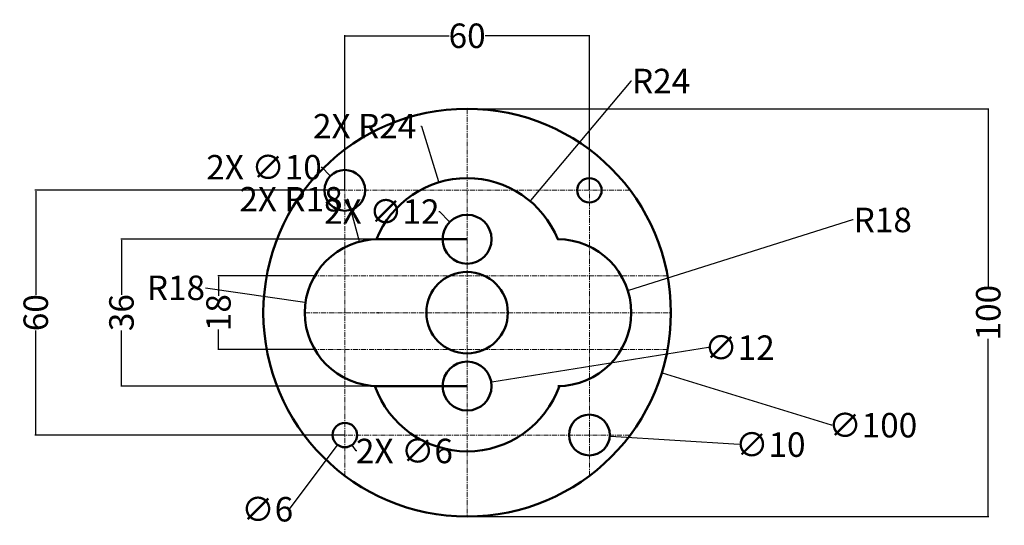
# Model space of a CAD drawing. Units: millimetres. Extents: x -18 to 223, y 11 to 135.
import ezdxf

# ---------------------------------------------------------------- set-up
doc = ezdxf.new("R2010")
doc.units = ezdxf.units.MM
doc.header["$MEASUREMENT"] = 0
doc.linetypes.add('CENTER', pattern=[2, 1.25, -0.25, 0.25, -0.25])
for name, color, linetype, lineweight in [('M-CNTR', 4, 'CENTER', 18), ('M-DIMS', 2, 'Continuous', 25), ('M-OUTL', 7, 'Continuous', 50)]:
    doc.layers.add(name, color=color, linetype=linetype, lineweight=lineweight)
doc.styles.get("Standard").update_dxf_attribs({"font": 'arial.ttf'})
doc.dimstyles.get("Standard").update_dxf_attribs({"dimtxt": 6, "dimasz": 0.18, "dimexe": 0.18, "dimexo": 0.0625, "dimgap": 0.09, "dimtad": 0, "dimtoh": 1, "dimdec": 0, "dimzin": 0, "dimdsep": 46, "dimtxsty": 'Standard', "dimcen": 0.09, "dimadec": 0, "dimazin": 0, "dimtfac": 1, "dimtdec": 0, "dimtofl": 0, "dimtmove": 0, "dimatfit": 3, "dimfxl": 1, "dimtolj": 1, "dimtzin": 0, "dimarcsym": 0})

# ---------------------------------------------------------------- blocks, each defined once
blk = doc.blocks.new('*D1')
at = {"layer": 'Defpoints', "color": 0, "transparency": 16777216}
for p in [(121.61, 131.04), (61.61, 93.14), (121.61, 93.14)]:
    blk.add_point(p, dxfattribs=at)
at = {"layer": 'M-DIMS', "color": 0, "lineweight": -2, "transparency": 16777216}
for p, q in [((61.61, 93.2), (61.61, 131.22)), ((61.79, 131.04), (87.22, 131.04)), ((121.43, 131.04), (96, 131.04)), ((121.61, 93.2), (121.61, 131.22))]:
    blk.add_line(p, q, dxfattribs=at)
at = {"layer": 'M-DIMS', "color": 0, "transparency": 16777216}
for points in [[(61.79, 131.07), (61.79, 131.01), (61.61, 131.04)], [(121.43, 131.07), (121.43, 131.01), (121.61, 131.04)]]:
    blk.add_solid(points, dxfattribs=at)
at = {"layer": 'M-DIMS', "color": 0, "transparency": 16777216, "insert": (91.61, 131.04), "char_height": 6, "attachment_point": 5}
blk.add_mtext('\\A1;60', dxfattribs=at)
blk = doc.blocks.new('*D2')
at = {"layer": 'Defpoints', "color": 0, "transparency": 16777216}
for p in [(43.84, 77.89), (139.39, 48.39)]:
    blk.add_point(p, dxfattribs=at)
at = {"layer": 'M-DIMS', "color": 0, "lineweight": -2, "transparency": 16777216}
for p, q in [((91.52, 63.14), (91.7, 63.14)), ((91.61, 63.05), (91.61, 63.23)), ((180.99, 35.55), (139.56, 48.34)), ((181.17, 35.55), (180.99, 35.55))]:
    blk.add_line(p, q, dxfattribs=at)
at = {"layer": 'M-DIMS', "color": 0, "transparency": 16777216}
blk.add_solid([(139.57, 48.36), (139.55, 48.31), (139.39, 48.39)], dxfattribs=at)
at = {"layer": 'M-DIMS', "color": 0, "transparency": 16777216, "insert": (191.14, 35.55), "char_height": 6, "attachment_point": 5}
blk.add_mtext('\\A1;∅100', dxfattribs=at)
blk = doc.blocks.new('*D3')
at = {"layer": 'Defpoints', "color": 0, "transparency": 16777216}
for p in [(91.61, 113.14), (91.61, 13.14), (219.47, 13.14)]:
    blk.add_point(p, dxfattribs=at)
at = {"layer": 'M-DIMS', "color": 0, "lineweight": -2, "transparency": 16777216}
for p, q in [((91.67, 113.14), (219.65, 113.14)), ((219.47, 112.96), (219.47, 69.56)), ((219.47, 13.32), (219.47, 56.71)), ((91.67, 13.14), (219.65, 13.14))]:
    blk.add_line(p, q, dxfattribs=at)
at = {"layer": 'M-DIMS', "color": 0, "transparency": 16777216}
for points in [[(219.44, 112.96), (219.5, 112.96), (219.47, 113.14)], [(219.44, 13.32), (219.5, 13.32), (219.47, 13.14)]]:
    blk.add_solid(points, dxfattribs=at)
at = {"layer": 'M-DIMS', "color": 0, "transparency": 16777216, "insert": (219.47, 63.14), "char_height": 6, "attachment_point": 5, "rotation": 90}
blk.add_mtext('\\A1;100', dxfattribs=at)
blk = doc.blocks.new('*D4')
at = {"layer": 'Defpoints', "color": 0, "transparency": 16777216}
for p in [(107.05, 90.51), (91.61, 72.14)]:
    blk.add_point(p, dxfattribs=at)
at = {"layer": 'M-DIMS', "color": 0, "lineweight": -2, "transparency": 16777216}
for p, q in [((131.79, 119.94), (107.17, 90.65)), ((131.97, 119.94), (131.79, 119.94)), ((91.52, 72.14), (91.7, 72.14)), ((91.61, 72.05), (91.61, 72.23))]:
    blk.add_line(p, q, dxfattribs=at)
at = {"layer": 'M-DIMS', "color": 0, "transparency": 16777216}
blk.add_solid([(107.14, 90.67), (107.19, 90.63), (107.05, 90.51)], dxfattribs=at)
at = {"layer": 'M-DIMS', "color": 0, "transparency": 16777216, "insert": (139.21, 119.94), "char_height": 6, "attachment_point": 5}
blk.add_mtext('\\A1;R24', dxfattribs=at)
blk = doc.blocks.new('*D5')
at = {"layer": 'Defpoints', "color": 0, "transparency": 16777216}
for p in [(51.98, 65.7), (69.79, 63.14)]:
    blk.add_point(p, dxfattribs=at)
at = {"layer": 'M-DIMS', "color": 0, "lineweight": -2, "transparency": 16777216}
for p, q in [((27.43, 69.23), (51.8, 65.72)), ((69.7, 63.14), (69.88, 63.14)), ((69.79, 63.05), (69.79, 63.23))]:
    blk.add_line(p, q, dxfattribs=at)
at = {"layer": 'M-DIMS', "color": 0, "transparency": 16777216}
blk.add_solid([(51.8, 65.75), (51.79, 65.7), (51.98, 65.7)], dxfattribs=at)
at = {"layer": 'M-DIMS', "color": 0, "transparency": 16777216, "insert": (20.17, 69.23), "char_height": 6, "attachment_point": 5}
blk.add_mtext('\\A1;R18', dxfattribs=at)
blk = doc.blocks.new('*D6')
at = {"layer": 'Defpoints', "color": 0, "transparency": 16777216}
for p in [(131.03, 68.54), (113.86, 63.14)]:
    blk.add_point(p, dxfattribs=at)
at = {"layer": 'M-DIMS', "color": 0, "lineweight": -2, "transparency": 16777216}
for p, q in [((186.14, 85.87), (131.2, 68.59)), ((186.32, 85.87), (186.14, 85.87)), ((113.77, 63.14), (113.95, 63.14)), ((113.86, 63.05), (113.86, 63.23))]:
    blk.add_line(p, q, dxfattribs=at)
at = {"layer": 'M-DIMS', "color": 0, "transparency": 16777216}
blk.add_solid([(131.19, 68.62), (131.21, 68.56), (131.03, 68.54)], dxfattribs=at)
at = {"layer": 'M-DIMS', "color": 0, "transparency": 16777216, "insert": (193.59, 85.87), "char_height": 6, "attachment_point": 5}
blk.add_mtext('\\A1;R18', dxfattribs=at)
blk = doc.blocks.new('*D7')
at = {"layer": 'Defpoints', "color": 0, "transparency": 16777216}
for p in [(63.4, 35.55), (59.82, 30.73)]:
    blk.add_point(p, dxfattribs=at)
at = {"layer": 'M-DIMS', "color": 0, "lineweight": -2, "transparency": 16777216}
for p, q in [((61.52, 33.14), (61.7, 33.14)), ((61.61, 33.05), (61.61, 33.23)), ((48.07, 14.94), (59.71, 30.59)), ((47.89, 14.94), (48.07, 14.94))]:
    blk.add_line(p, q, dxfattribs=at)
at = {"layer": 'M-DIMS', "color": 0, "transparency": 16777216}
blk.add_solid([(59.69, 30.61), (59.74, 30.57), (59.82, 30.73)], dxfattribs=at)
at = {"layer": 'M-DIMS', "color": 0, "transparency": 16777216, "insert": (42.57, 14.94), "char_height": 6, "attachment_point": 5}
blk.add_mtext('\\A1;∅6', dxfattribs=at)
blk = doc.blocks.new('*D8')
at = {"layer": 'Defpoints', "color": 0, "transparency": 16777216}
for p in [(116.62, 33.46), (126.6, 32.82)]:
    blk.add_point(p, dxfattribs=at)
at = {"layer": 'M-DIMS', "color": 0, "lineweight": -2, "transparency": 16777216}
for p, q in [((121.52, 33.14), (121.7, 33.14)), ((121.61, 33.05), (121.61, 33.23)), ((158.37, 30.79), (126.78, 32.81))]:
    blk.add_line(p, q, dxfattribs=at)
at = {"layer": 'M-DIMS', "color": 0, "transparency": 16777216}
blk.add_solid([(126.78, 32.84), (126.78, 32.78), (126.6, 32.82)], dxfattribs=at)
at = {"layer": 'M-DIMS', "color": 0, "transparency": 16777216, "insert": (166.01, 30.79), "char_height": 6, "attachment_point": 5}
blk.add_mtext('\\A1;∅10', dxfattribs=at)
blk = doc.blocks.new('*D9')
at = {"layer": 'Defpoints', "color": 0, "transparency": 16777216}
for p in [(97.54, 46.08), (85.68, 44.2)]:
    blk.add_point(p, dxfattribs=at)
at = {"layer": 'M-DIMS', "color": 0, "lineweight": -2, "transparency": 16777216}
for p, q in [((150.83, 54.57), (97.71, 46.11)), ((91.52, 45.14), (91.7, 45.14)), ((91.61, 45.05), (91.61, 45.23))]:
    blk.add_line(p, q, dxfattribs=at)
at = {"layer": 'M-DIMS', "color": 0, "transparency": 16777216}
blk.add_solid([(97.71, 46.14), (97.72, 46.08), (97.54, 46.08)], dxfattribs=at)
at = {"layer": 'M-DIMS', "color": 0, "transparency": 16777216, "insert": (158.45, 54.57), "char_height": 6, "attachment_point": 5}
blk.add_mtext('\\A1;∅12', dxfattribs=at)
blk = doc.blocks.new('*D10')
at = {"layer": 'Defpoints', "color": 0, "transparency": 16777216}
for p in [(54.2, 72.14), (30.61, 54.14), (54.2, 54.14)]:
    blk.add_point(p, dxfattribs=at)
at = {"layer": 'M-DIMS', "color": 0, "lineweight": -2, "transparency": 16777216}
for p, q in [((54.14, 72.14), (30.43, 72.14)), ((30.61, 71.96), (30.61, 67.25)), ((30.61, 54.32), (30.61, 59.03)), ((54.14, 54.14), (30.43, 54.14))]:
    blk.add_line(p, q, dxfattribs=at)
at = {"layer": 'M-DIMS', "color": 0, "transparency": 16777216}
for points in [[(30.58, 71.96), (30.64, 71.96), (30.61, 72.14)], [(30.58, 54.32), (30.64, 54.32), (30.61, 54.14)]]:
    blk.add_solid(points, dxfattribs=at)
at = {"layer": 'M-DIMS', "color": 0, "transparency": 16777216, "insert": (30.61, 63.14), "char_height": 6, "attachment_point": 5, "rotation": 90}
blk.add_mtext('\\A1;18', dxfattribs=at)
blk = doc.blocks.new('*D11')
at = {"layer": 'Defpoints', "color": 0, "transparency": 16777216}
for p in [(69.36, 81.13), (6.8, 45.14), (69.79, 45.14)]:
    blk.add_point(p, dxfattribs=at)
at = {"layer": 'M-DIMS', "color": 0, "lineweight": -2, "transparency": 16777216}
for p, q in [((69.3, 81.13), (6.62, 81.13)), ((6.8, 80.95), (6.8, 67.52)), ((6.8, 45.32), (6.8, 58.75)), ((69.73, 45.14), (6.62, 45.14))]:
    blk.add_line(p, q, dxfattribs=at)
at = {"layer": 'M-DIMS', "color": 0, "transparency": 16777216}
for points in [[(6.77, 80.95), (6.83, 80.95), (6.8, 81.13)], [(6.77, 45.32), (6.83, 45.32), (6.8, 45.14)]]:
    blk.add_solid(points, dxfattribs=at)
at = {"layer": 'M-DIMS', "color": 0, "transparency": 16777216, "insert": (6.8, 63.14), "char_height": 6, "attachment_point": 5, "rotation": 90}
blk.add_mtext('\\A1;36', dxfattribs=at)
blk = doc.blocks.new('*D12')
at = {"layer": 'Defpoints', "color": 0, "transparency": 16777216}
for p in [(61.61, 93.14), (-14.23, 33.14), (61.52, 33.14)]:
    blk.add_point(p, dxfattribs=at)
at = {"layer": 'M-DIMS', "color": 0, "lineweight": -2, "transparency": 16777216}
for p, q in [((61.55, 93.14), (-14.41, 93.14)), ((-14.23, 92.96), (-14.23, 67.53)), ((-14.23, 33.32), (-14.23, 58.75)), ((61.46, 33.14), (-14.41, 33.14))]:
    blk.add_line(p, q, dxfattribs=at)
at = {"layer": 'M-DIMS', "color": 0, "transparency": 16777216}
for points in [[(-14.26, 92.96), (-14.2, 92.96), (-14.23, 93.14)], [(-14.26, 33.32), (-14.2, 33.32), (-14.23, 33.14)]]:
    blk.add_solid(points, dxfattribs=at)
at = {"layer": 'M-DIMS', "color": 0, "transparency": 16777216, "insert": (-14.23, 63.14), "char_height": 6, "attachment_point": 5, "rotation": 90}
blk.add_mtext('\\A1;60', dxfattribs=at)
blk = doc.blocks.new('INNER-HOLE-D12')
blk.add_circle((6, 6), 6)
blk = doc.blocks.new('MOUNT-HOLE-D10')
blk.add_circle((5, 5), 5)
blk = doc.blocks.new('MOUNT-HOLE-D6')
blk.add_circle((3, 3), 3)
blk = doc.blocks.new('*D16')
at = {"layer": 'Defpoints', "color": 0, "transparency": 16777216}
for p in [(84.6, 95.09), (91.61, 72.14)]:
    blk.add_point(p, dxfattribs=at)
at = {"layer": 'M-DIMS', "color": 0, "lineweight": -2, "transparency": 16777216}
for p, q in [((80.22, 108.87), (80.4, 108.87)), ((80.4, 108.87), (84.55, 95.27)), ((91.52, 72.14), (91.7, 72.14)), ((91.61, 72.05), (91.61, 72.23))]:
    blk.add_line(p, q, dxfattribs=at)
at = {"layer": 'M-DIMS', "color": 0, "transparency": 16777216}
blk.add_solid([(84.58, 95.27), (84.52, 95.26), (84.6, 95.09)], dxfattribs=at)
at = {"layer": 'M-DIMS', "color": 0, "transparency": 16777216, "insert": (66.47, 108.87), "char_height": 6, "attachment_point": 5}
blk.add_mtext('\\A1;2X R24', dxfattribs=at)
blk = doc.blocks.new('*D17')
at = {"layer": 'Defpoints', "color": 0, "transparency": 16777216}
for p in [(65.13, 80.53), (69.79, 63.14)]:
    blk.add_point(p, dxfattribs=at)
at = {"layer": 'M-DIMS', "color": 0, "lineweight": -2, "transparency": 16777216}
for p, q in [((62.16, 90.96), (62.34, 90.96)), ((62.34, 90.96), (65.09, 80.7)), ((69.7, 63.14), (69.88, 63.14)), ((69.79, 63.05), (69.79, 63.23))]:
    blk.add_line(p, q, dxfattribs=at)
at = {"layer": 'M-DIMS', "color": 0, "transparency": 16777216}
blk.add_solid([(65.12, 80.71), (65.06, 80.69), (65.13, 80.53)], dxfattribs=at)
at = {"layer": 'M-DIMS', "color": 0, "transparency": 16777216, "insert": (48.4, 90.96), "char_height": 6, "attachment_point": 5}
blk.add_mtext('\\A1;2X R18', dxfattribs=at)
blk = doc.blocks.new('*D18')
at = {"layer": 'Defpoints', "color": 0, "transparency": 16777216}
for p in [(87.37, 85.38), (95.85, 76.9)]:
    blk.add_point(p, dxfattribs=at)
at = {"layer": 'M-DIMS', "color": 0, "lineweight": -2, "transparency": 16777216}
for p, q in [((84.64, 87.93), (84.82, 87.93)), ((84.82, 87.93), (87.24, 85.51)), ((91.52, 81.14), (91.7, 81.14)), ((91.61, 81.05), (91.61, 81.23))]:
    blk.add_line(p, q, dxfattribs=at)
at = {"layer": 'M-DIMS', "color": 0, "transparency": 16777216}
blk.add_solid([(87.26, 85.53), (87.22, 85.49), (87.37, 85.38)], dxfattribs=at)
at = {"layer": 'M-DIMS', "color": 0, "transparency": 16777216, "insert": (70.68, 87.93), "char_height": 6, "attachment_point": 5}
blk.add_mtext('\\A1;2X ∅12', dxfattribs=at)
blk = doc.blocks.new('*D19')
at = {"layer": 'Defpoints', "color": 0, "transparency": 16777216}
for p in [(58.07, 96.67), (65.15, 89.6)]:
    blk.add_point(p, dxfattribs=at)
at = {"layer": 'M-DIMS', "color": 0, "lineweight": -2, "transparency": 16777216}
for p, q in [((55.77, 98.8), (55.95, 98.8)), ((55.95, 98.8), (57.95, 96.8)), ((61.52, 93.14), (61.7, 93.14)), ((61.61, 93.05), (61.61, 93.23))]:
    blk.add_line(p, q, dxfattribs=at)
at = {"layer": 'M-DIMS', "color": 0, "transparency": 16777216}
blk.add_solid([(57.97, 96.82), (57.93, 96.78), (58.07, 96.67)], dxfattribs=at)
at = {"layer": 'M-DIMS', "color": 0, "transparency": 16777216, "insert": (41.79, 98.8), "char_height": 6, "attachment_point": 5}
blk.add_mtext('\\A1;2X ∅10', dxfattribs=at)
blk = doc.blocks.new('*D20')
at = {"layer": 'Defpoints', "color": 0, "transparency": 16777216}
for p in [(59.87, 35.58), (63.35, 30.7)]:
    blk.add_point(p, dxfattribs=at)
at = {"layer": 'M-DIMS', "color": 0, "lineweight": -2, "transparency": 16777216}
for p, q in [((61.52, 33.14), (61.7, 33.14)), ((61.61, 33.05), (61.61, 33.23)), ((64.39, 29.23), (63.45, 30.55)), ((64.57, 29.23), (64.39, 29.23))]:
    blk.add_line(p, q, dxfattribs=at)
at = {"layer": 'M-DIMS', "color": 0, "transparency": 16777216}
blk.add_solid([(63.48, 30.57), (63.43, 30.53), (63.35, 30.7)], dxfattribs=at)
at = {"layer": 'M-DIMS', "color": 0, "transparency": 16777216, "insert": (76.23, 29.23), "char_height": 6, "attachment_point": 5}
blk.add_mtext('\\A1;2X ∅6', dxfattribs=at)

msp = doc.modelspace()

# ---------------------------------------------------------------- linework, layer by layer
at = {"layer": 'M-CNTR'}
for p, q in [((61.61, 23.14), (61.61, 103.14)), ((121.61, 23.14), (121.61, 103.14)), ((131.61, 93.14), (51.61, 93.14)), ((140.79, 72.14), (54.2, 72.14)), ((140.79, 54.14), (54.2, 54.14)), ((131.61, 33.14), (51.61, 33.14))]:
    msp.add_line(p, q, dxfattribs=at)
for points in [[(91.61, 113.14), (91.61, 63.14), (91.61, 13.14)], [(51.79, 63.14), (91.61, 63.14), (141.61, 63.14)]]:
    msp.add_lwpolyline(points, dxfattribs=at)
at = {"layer": 'M-OUTL'}
for points in [[(113.86, 45.14, 1), (113.86, 81.14, 0.674285), (69.36, 81.13)], [(91.61, 81.14), (69.79, 81.14, 1), (69.79, 45.14)]]:
    msp.add_lwpolyline(points, format="xyb", dxfattribs=at)
for points in [[(91.61, 45.14), (68.98, 45.14)], [(114.24, 45.14), (113.86, 45.14)]]:
    msp.add_lwpolyline(points, dxfattribs=at)
for radius in [50, 10]:
    msp.add_circle((91.61, 63.14), radius, dxfattribs=at)
msp.add_arc((91.61, 53.14), 24, 199.4243, 340.5288, dxfattribs=at)

# ---------------------------------------------------------------- block references
for name, p in [('MOUNT-HOLE-D10', (56.61, 88.14)), ('MOUNT-HOLE-D6', (118.61, 90.14)), ('INNER-HOLE-D12', (85.61, 75.14)), ('INNER-HOLE-D12', (85.61, 39.14)), ('MOUNT-HOLE-D10', (116.61, 28.14)), ('MOUNT-HOLE-D6', (58.61, 30.14))]:
    msp.add_blockref(name, p, dxfattribs=at)

# ---------------------------------------------------------------- dimensions: what is measured, and where the dimension line sits
at = {"layer": 'M-DIMS'}
dim = msp.add_linear_dim(base=(121.61, 131.04), p1=(61.61, 93.14), p2=(121.61, 93.14), dimstyle='Standard', override={"dimclrd": 0, "dimclre": 0, "dimclrt": 0}, dxfattribs=at)
dim.commit()
dim.dimension.update_dxf_attribs({"geometry": '*D1', "text_midpoint": (91.61, 131.04)})
for center, mpoint, picture, middle in [((91.61, 72.14), (107.05, 90.51), '*D4', (139.21, 119.94)), ((113.86, 63.14), (131.03, 68.54), '*D6', (193.59, 85.87)), ((69.79, 63.14), (51.98, 65.7), '*D5', (27.43, 69.23))]:
    dim = msp.add_radius_dim(center=center, mpoint=mpoint, dimstyle='Standard', override={"dimclrd": 0, "dimclre": 0, "dimclrt": 0}, dxfattribs=at)
    dim.commit()
    dim.dimension.update_dxf_attribs({"geometry": picture, "text_midpoint": middle, "dimtype": 164})
for center, mpoint, picture, middle in [((91.61, 72.14), (84.6, 95.09), '*D16', (66.47, 108.87)), ((69.79, 63.14), (65.13, 80.53), '*D17', (48.4, 90.96))]:
    dim = msp.add_radius_dim(center=center, mpoint=mpoint, text='2X <>', dimstyle='Standard', override={"dimdec": 0, "dimlfac": 1, "dimrnd": 0, "dimzin": 0, "dimdsep": 46, "dimlunit": 2}, dxfattribs=at)
    dim.commit()
    dim.dimension.update_dxf_attribs({"geometry": picture, "text_midpoint": middle, "dimtype": 164})
for base, p1, p2, picture, middle in [((219.47, 13.14), (91.61, 113.14), (91.61, 13.14), '*D3', (219.47, 63.14)), ((-14.23, 33.14), (61.61, 93.14), (61.52, 33.14), '*D12', (-14.23, 63.14)), ((6.8, 45.14), (69.36, 81.13), (69.79, 45.14), '*D11', (6.8, 63.14)), ((30.61, 54.14), (54.2, 72.14), (54.2, 54.14), '*D10', (30.61, 63.14))]:
    dim = msp.add_linear_dim(base=base, p1=p1, p2=p2, angle=90, dimstyle='Standard', override={"dimclrd": 0, "dimclre": 0, "dimclrt": 0}, dxfattribs=at)
    dim.commit()
    dim.dimension.update_dxf_attribs({"geometry": picture, "text_midpoint": middle})
for p1, p2, picture, middle in [((65.15, 89.6), (58.07, 96.67), '*D19', (41.79, 98.8)), ((95.85, 76.9), (87.37, 85.38), '*D18', (70.68, 87.93)), ((59.87, 35.58), (63.35, 30.7), '*D20', (76.23, 29.23))]:
    dim = msp.add_diameter_dim_2p(p1=p1, p2=p2, text='2X <>', dimstyle='Standard', override={"dimdec": 0, "dimlfac": 1, "dimrnd": 0, "dimzin": 0, "dimdsep": 46, "dimlunit": 2}, dxfattribs=at)
    dim.commit()
    dim.dimension.update_dxf_attribs({"geometry": picture, "text_midpoint": middle, "dimtype": 163})
for p1, p2, picture, middle in [((43.84, 77.89), (139.39, 48.39), '*D2', (191.14, 35.55)), ((85.68, 44.2), (97.54, 46.08), '*D9', (150.83, 54.57)), ((63.4, 35.55), (59.82, 30.73), '*D7', (42.57, 14.94)), ((116.62, 33.46), (126.6, 32.82), '*D8', (158.37, 30.79))]:
    dim = msp.add_diameter_dim_2p(p1=p1, p2=p2, dimstyle='Standard', override={"dimclrd": 0, "dimclre": 0, "dimclrt": 0}, dxfattribs=at)
    dim.commit()
    dim.dimension.update_dxf_attribs({"geometry": picture, "text_midpoint": middle, "dimtype": 163})

doc.saveas('drawing.dxf')
